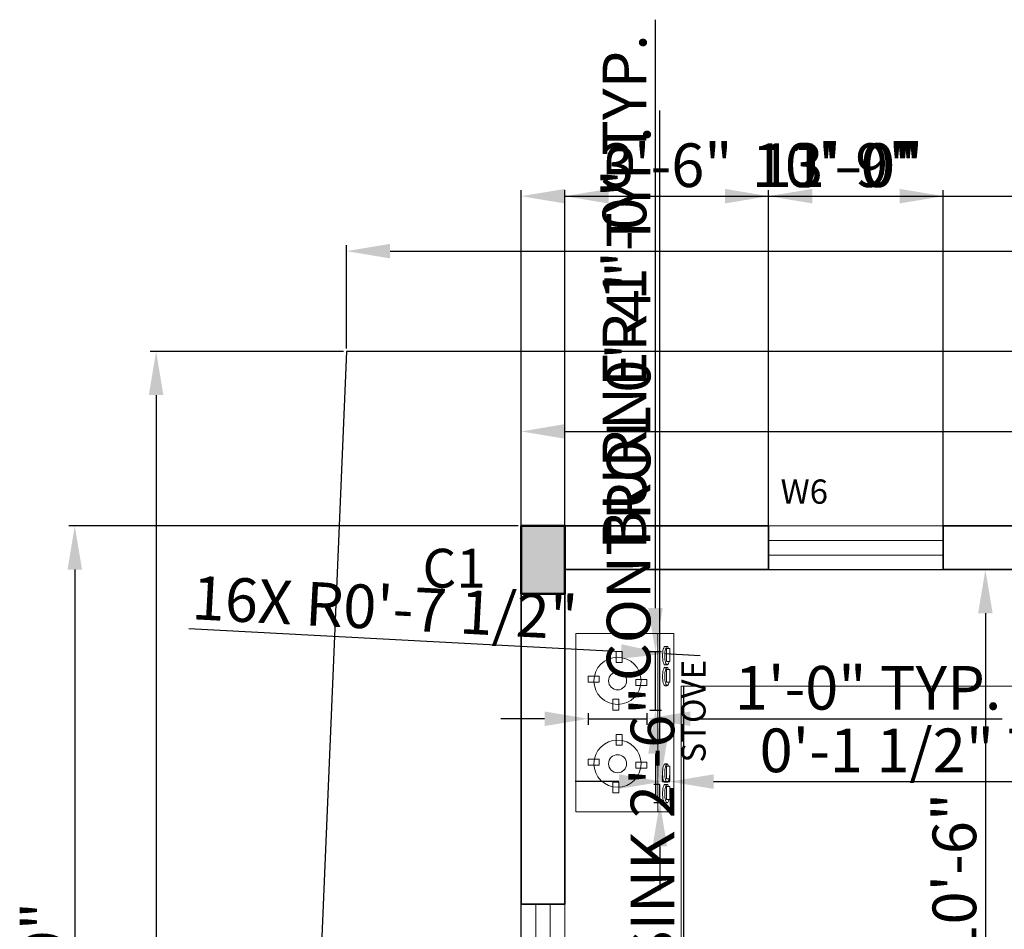
# Model space of a CAD drawing. Units: inches. Extents: x 2621 to 6190, y 513 to 1320.
# Tile 4 of 11: x 2675 to 2878, y 1003 to 1190. Entities that reach past the tile are written whole.
import ezdxf

# ---------------------------------------------------------------- set-up
doc = ezdxf.new("R2010")
doc.units = ezdxf.units.IN
for name, color, linetype, lineweight in [('A-ANNO-DIMS', 5, 'Continuous', 18), ('A-ANNO-TEXT', 7, 'Continuous', 18), ('A-EQPM', 30, 'Continuous', 13), ('A-FLOR-CASE', 30, 'Continuous', 18), ('A-WALL', 7, 'Continuous', 35), ('C-PROP', 7, 'Continuous', 25), ('columns', 2, 'Continuous', 50), ('S-COLS-IDEN', 2, 'Continuous', 25), ('S-COLS-PATT', 2, 'Continuous', 13), ('window', 172, 'Continuous', 18)]:
    doc.layers.add(name, color=color, linetype=linetype, lineweight=lineweight)
doc.styles.get("Standard").update_dxf_attribs({"font": 'arial.ttf'})
doc.dimstyles.new('ISO-25', dxfattribs={"dimtxt": 9, "dimasz": 9, "dimexe": 1.25, "dimexo": 0.625, "dimtad": 1, "dimlunit": 3, "dimtxsty": 'Standard', "dimcen": 2.5, "dimadec": 0, "dimazin": 0, "dimtfac": 1, "dimtmove": 0, "dimatfit": 3, "dimfxl": 1, "dimarcsym": 0})

# ---------------------------------------------------------------- blocks, each defined once
blk = doc.blocks.new('*D18')
at = {"layer": 'A-ANNO-DIMS', "color": 0, "lineweight": -2, "transparency": 16777216}
for p, q in [((2820.57, 1076.89), (2875.3, 1076.89)), ((2874.05, 1067.89), (2874.05, 959.89)), ((2820.57, 950.89), (2875.3, 950.89))]:
    blk.add_line(p, q, dxfattribs=at)
at = {"layer": 'A-ANNO-DIMS', "color": 0, "transparency": 16777216}
for points in [[(2872.55, 1067.89), (2875.55, 1067.89), (2874.05, 1076.89)], [(2872.55, 959.89), (2875.55, 959.89), (2874.05, 950.89)]]:
    blk.add_solid(points, dxfattribs=at)
at = {"layer": 'Defpoints', "color": 0, "transparency": 16777216}
for p in [(2819.94, 1076.89), (2819.94, 950.89), (2874.05, 950.89)]:
    blk.add_point(p, dxfattribs=at)
at = {"layer": 'A-ANNO-DIMS', "color": 0, "transparency": 16777216, "insert": (2868.83, 1013.89), "char_height": 9, "attachment_point": 5, "rotation": 90}
blk.add_mtext('10\'-6"', dxfattribs=at)
blk = doc.blocks.new('*D36')
at = {"layer": 'A-ANNO-DIMS', "color": 0, "lineweight": -2, "transparency": 16777216}
for p, q in [((2778.38, 1086.51), (2778.38, 1106.64)), ((3222.38, 1086.51), (3222.38, 1106.64)), ((2787.38, 1105.39), (3213.38, 1105.39))]:
    blk.add_line(p, q, dxfattribs=at)
at = {"layer": 'A-ANNO-DIMS', "color": 0, "transparency": 16777216}
for points in [[(2787.38, 1106.89), (2787.38, 1103.89), (2778.38, 1105.39)], [(3213.38, 1106.89), (3213.38, 1103.89), (3222.38, 1105.39)]]:
    blk.add_solid(points, dxfattribs=at)
at = {"layer": 'Defpoints', "color": 0, "transparency": 16777216}
for p in [(3222.38, 1105.39), (2778.38, 1085.89), (3222.38, 1085.89)]:
    blk.add_point(p, dxfattribs=at)
at = {"layer": 'A-ANNO-DIMS', "color": 0, "transparency": 16777216, "insert": (3000.38, 1110.61), "char_height": 9, "attachment_point": 5}
blk.add_mtext("37'", dxfattribs=at)
blk = doc.blocks.new('*D38')
at = {"layer": 'A-ANNO-DIMS', "color": 0, "lineweight": -2, "transparency": 16777216}
for p, q in [((2742.38, 1122.51), (2742.38, 1143.81)), ((2751.38, 1142.56), (3249.38, 1142.56)), ((3258.38, 1122.51), (3258.38, 1143.81))]:
    blk.add_line(p, q, dxfattribs=at)
at = {"layer": 'A-ANNO-DIMS', "color": 0, "transparency": 16777216}
for points in [[(2751.38, 1144.06), (2751.38, 1141.06), (2742.38, 1142.56)], [(3249.38, 1144.06), (3249.38, 1141.06), (3258.38, 1142.56)]]:
    blk.add_solid(points, dxfattribs=at)
at = {"layer": 'Defpoints', "color": 0, "transparency": 16777216}
for p in [(3258.38, 1142.56), (2742.38, 1121.89), (3258.38, 1121.89)]:
    blk.add_point(p, dxfattribs=at)
at = {"layer": 'A-ANNO-DIMS', "color": 0, "transparency": 16777216, "insert": (3000.38, 1147.79), "char_height": 9, "attachment_point": 5}
blk.add_mtext("43'", dxfattribs=at)
blk = doc.blocks.new('*D40')
at = {"layer": 'A-ANNO-DIMS', "color": 0, "lineweight": -2, "transparency": 16777216}
for p, q in [((2741.76, 1121.89), (2701.89, 1121.89)), ((2703.14, 1112.89), (2703.14, 561.89)), ((2717.76, 552.89), (2701.89, 552.89))]:
    blk.add_line(p, q, dxfattribs=at)
at = {"layer": 'A-ANNO-DIMS', "color": 0, "transparency": 16777216}
for points in [[(2701.64, 1112.89), (2704.64, 1112.89), (2703.14, 1121.89)], [(2701.64, 561.89), (2704.64, 561.89), (2703.14, 552.89)]]:
    blk.add_solid(points, dxfattribs=at)
at = {"layer": 'Defpoints', "color": 0, "transparency": 16777216}
for p in [(2742.38, 1121.89), (2703.14, 552.89), (2718.38, 552.89)]:
    blk.add_point(p, dxfattribs=at)
at = {"layer": 'A-ANNO-DIMS', "color": 0, "transparency": 16777216, "insert": (2697.94, 837.39), "char_height": 9, "attachment_point": 5, "rotation": 90}
blk.add_mtext('47\'-5"', dxfattribs=at)
blk = doc.blocks.new('WIN-VENT-24IN')
for p, q in [((9, 24), (0, 24)), ((0, 24), (0, 0)), ((3, 24), (3, 0)), ((6, 24), (6, 0)), ((9, 0), (9, 24)), ((0, 0), (9, 0))]:
    blk.add_line(p, q)
blk = doc.blocks.new('COOKTOP-BURNER')
for p, q in [((6.96, 12.04), (5.73, 12.04)), ((5.73, 12.04), (5.73, 9.81)), ((6.96, 9.81), (6.96, 12.04)), ((5.73, 9.81), (6.96, 9.81)), ((2.23, 6.96), (0, 6.96)), ((0, 6.96), (0, 5.73)), ((2.23, 5.73), (2.23, 6.96)), ((12.04, 6.31), (9.81, 6.31)), ((9.81, 6.31), (9.81, 5.08)), ((12.04, 5.08), (12.04, 6.31)), ((0, 5.73), (2.23, 5.73)), ((9.81, 5.08), (12.04, 5.08)), ((5.08, 2.23), (5.08, 0)), ((6.31, 2.23), (5.08, 2.23)), ((6.31, 0), (6.31, 2.23)), ((5.08, 0), (6.31, 0))]:
    blk.add_line(p, q)
for radius in [4.86, 1.86]:
    blk.add_circle((6.02, 6.02), radius)
blk = doc.blocks.new('COOKTOP-CONTROL')
for p, q in [((0.44, 3.79), (0.92, 3.78)), ((0.83, 3.35), (1.52, 3.35)), ((0.83, 0.69), (0.83, 3.35)), ((1.52, 3.35), (1.52, 0.69)), ((0.49, 0), (0.92, 0)), ((1.52, 0.69), (0.83, 0.69))]:
    blk.add_line(p, q)
for centre, radius, start, end in [((7.32, 1.89), 7.32, 173.9017, 180), ((3.91, 2.25), 3.89, 165.5369, 173.9017), ((1.79, 2.8), 1.7, 148.0894, 165.5369), ((0.49, 3.61), 0.166, 90, 148.0894), ((7.76, 1.89), 7.32, 173.9017, 180), ((4.35, 2.25), 3.89, 165.5369, 173.9017), ((0.49, 3.61), 0.166, 72.0546, 90), ((2.23, 2.8), 1.7, 148.0894, 165.5369), ((0.92, 3.61), 0.166, 90, 148.0894), ((0.92, 3.61), 0.166, 31.9106, 90), ((-0.38, 2.8), 1.7, 18.9155, 31.9106), ((7.32, 1.89), 7.32, 180, 186.0983), ((3.91, 1.53), 3.89, 186.0983, 194.4631), ((1.79, 0.98), 1.7, 194.4631, 211.9106), ((0.49, 0.17), 0.166, 211.9106, 270), ((7.76, 1.89), 7.32, 180, 186.0983), ((4.35, 1.53), 3.89, 186.0983, 194.4631), ((2.23, 0.98), 1.7, 194.4631, 211.9106), ((0.92, 0.17), 0.166, 211.9106, 270), ((0.92, 0.17), 0.166, 270, 328.0894), ((-0.38, 0.98), 1.7, 328.0894, 345.5369), ((-2.5, 1.53), 3.89, 345.5369, 347.5389)]:
    blk.add_arc(centre, radius, start, end)
blk = doc.blocks.new('*D67')
at = {"layer": 'A-ANNO-DIMS', "color": 0, "lineweight": -2, "transparency": 16777216}
for p, q in [((2806.96, 1041.61), (2806.96, 1171.58)), ((2806.9, 1032.61), (2805.71, 1032.61)), ((2806.96, 1028.83), (2806.96, 1032.61)), ((2806.9, 1028.83), (2805.71, 1028.83)), ((2806.96, 1019.83), (2806.96, 1010.83))]:
    blk.add_line(p, q, dxfattribs=at)
at = {"layer": 'A-ANNO-DIMS', "color": 0, "transparency": 16777216}
for points in [[(2805.46, 1041.61), (2808.46, 1041.61), (2806.96, 1032.61)], [(2805.46, 1019.83), (2808.46, 1019.83), (2806.96, 1028.83)]]:
    blk.add_solid(points, dxfattribs=at)
at = {"layer": 'Defpoints', "color": 0, "transparency": 16777216}
for p in [(2806.96, 1032.61), (2807.53, 1032.61), (2807.53, 1028.83)]:
    blk.add_point(p, dxfattribs=at)
at = {"layer": 'A-ANNO-DIMS', "color": 0, "transparency": 16777216, "insert": (2801.68, 1111.1), "char_height": 9, "attachment_point": 5, "rotation": 90}
blk.add_mtext('CONTROL 0\'-4" TYP.', dxfattribs=at)
blk = doc.blocks.new('*D68')
at = {"layer": 'A-ANNO-DIMS', "color": 0, "lineweight": -2, "transparency": 16777216}
for p, q in [((2798.53, 1033.18), (2789.53, 1033.18)), ((2807.53, 1033.24), (2807.53, 1034.43)), ((2807.53, 1033.18), (2809.04, 1033.18)), ((2809.04, 1033.24), (2809.04, 1034.43)), ((2818.04, 1033.18), (2904.12, 1033.18))]:
    blk.add_line(p, q, dxfattribs=at)
at = {"layer": 'A-ANNO-DIMS', "color": 0, "transparency": 16777216}
for points in [[(2798.53, 1034.68), (2798.53, 1031.68), (2807.53, 1033.18)], [(2818.04, 1034.68), (2818.04, 1031.68), (2809.04, 1033.18)]]:
    blk.add_solid(points, dxfattribs=at)
at = {"layer": 'Defpoints', "color": 0, "transparency": 16777216}
for p in [(2809.04, 1033.18), (2807.53, 1032.61), (2809.04, 1032.61)]:
    blk.add_point(p, dxfattribs=at)
at = {"layer": 'A-ANNO-DIMS', "color": 0, "transparency": 16777216, "insert": (2865.58, 1038.46), "char_height": 9, "attachment_point": 5}
blk.add_mtext('0\'-1 1/2" TYP.', dxfattribs=at)
blk = doc.blocks.new('*D69')
at = {"layer": 'A-ANNO-DIMS', "color": 0, "lineweight": -2, "transparency": 16777216}
for p, q in [((2806.06, 1068.98), (2806.06, 1190.28)), ((2804.88, 1059.98), (2807.31, 1059.98)), ((2806.06, 1047.94), (2806.06, 1059.98)), ((2804.88, 1047.94), (2807.31, 1047.94)), ((2806.06, 1038.94), (2806.06, 1029.94))]:
    blk.add_line(p, q, dxfattribs=at)
at = {"layer": 'A-ANNO-DIMS', "color": 0, "transparency": 16777216}
for points in [[(2804.56, 1068.98), (2807.56, 1068.98), (2806.06, 1059.98)], [(2804.56, 1038.94), (2807.56, 1038.94), (2806.06, 1047.94)]]:
    blk.add_solid(points, dxfattribs=at)
at = {"layer": 'Defpoints', "color": 0, "transparency": 16777216}
for p in [(2804.26, 1059.98), (2806.06, 1059.98), (2804.26, 1047.94)]:
    blk.add_point(p, dxfattribs=at)
at = {"layer": 'A-ANNO-DIMS', "color": 0, "transparency": 16777216, "insert": (2800.84, 1134.13), "char_height": 9, "attachment_point": 5, "rotation": 90}
blk.add_mtext('BURNER 1\'-0" TYP.', dxfattribs=at)
blk = doc.blocks.new('*D70')
at = {"layer": 'A-ANNO-DIMS', "color": 0, "lineweight": -2, "transparency": 16777216}
for p, q in [((2792.22, 1047.32), (2792.22, 1044.89)), ((2804.26, 1047.32), (2804.26, 1044.89)), ((2783.22, 1046.14), (2774.22, 1046.14)), ((2792.22, 1046.14), (2804.26, 1046.14)), ((2813.26, 1046.14), (2877.52, 1046.14))]:
    blk.add_line(p, q, dxfattribs=at)
at = {"layer": 'A-ANNO-DIMS', "color": 0, "transparency": 16777216}
for points in [[(2783.22, 1047.64), (2783.22, 1044.64), (2792.22, 1046.14)], [(2813.26, 1047.64), (2813.26, 1044.64), (2804.26, 1046.14)]]:
    blk.add_solid(points, dxfattribs=at)
at = {"layer": 'Defpoints', "color": 0, "transparency": 16777216}
for p in [(2792.22, 1047.94), (2804.26, 1047.94), (2804.26, 1046.14)]:
    blk.add_point(p, dxfattribs=at)
at = {"layer": 'A-ANNO-DIMS', "color": 0, "transparency": 16777216, "insert": (2849.89, 1051.36), "char_height": 9, "attachment_point": 5}
blk.add_mtext('1\'-0" TYP.', dxfattribs=at)
blk = doc.blocks.new('*D77')
at = {"layer": 'A-ANNO-DIMS', "color": 0, "lineweight": -2, "transparency": 16777216}
for p, q in [((2811.88, 985.99), (2811.88, 1052.96)), ((2808.01, 985.99), (2813.13, 985.99)), ((2811.88, 964.99), (2811.88, 976.99)), ((2808.01, 955.99), (2813.13, 955.99))]:
    blk.add_line(p, q, dxfattribs=at)
at = {"layer": 'A-ANNO-DIMS', "color": 0, "transparency": 16777216}
for points in [[(2810.38, 976.99), (2813.38, 976.99), (2811.88, 985.99)], [(2810.38, 964.99), (2813.38, 964.99), (2811.88, 955.99)]]:
    blk.add_solid(points, dxfattribs=at)
at = {"layer": 'Defpoints', "color": 0, "transparency": 16777216}
for p in [(2807.38, 985.99), (2811.88, 985.99), (2807.38, 955.99)]:
    blk.add_point(p, dxfattribs=at)
at = {"layer": 'A-ANNO-DIMS', "color": 0, "transparency": 16777216, "insert": (2806.6, 1023.98), "char_height": 9, "attachment_point": 5, "rotation": 90}
blk.add_mtext('SINK 2\'-6"', dxfattribs=at)
blk = doc.blocks.new('*D79')
at = {"layer": 'A-ANNO-DIMS', "color": 0, "lineweight": -2, "transparency": 16777216}
for p, q in [((2778.38, 1086.51), (2778.38, 1155.14)), ((2907.38, 1086.51), (2907.38, 1155.14)), ((2787.38, 1153.89), (2898.38, 1153.89))]:
    blk.add_line(p, q, dxfattribs=at)
at = {"layer": 'A-ANNO-DIMS', "color": 0, "transparency": 16777216}
for points in [[(2787.38, 1155.39), (2787.38, 1152.39), (2778.38, 1153.89)], [(2898.38, 1155.39), (2898.38, 1152.39), (2907.38, 1153.89)]]:
    blk.add_solid(points, dxfattribs=at)
at = {"layer": 'Defpoints', "color": 0, "transparency": 16777216}
for p in [(2907.38, 1153.89), (2778.38, 1085.89), (2907.38, 1085.89)]:
    blk.add_point(p, dxfattribs=at)
at = {"layer": 'A-ANNO-DIMS', "color": 0, "transparency": 16777216, "insert": (2842.88, 1159.11), "char_height": 9, "attachment_point": 5}
blk.add_mtext('10\'-9"', dxfattribs=at)
blk = doc.blocks.new('*D81')
at = {"layer": 'A-ANNO-DIMS', "color": 0, "lineweight": -2, "transparency": 16777216}
for p, q in [((2777.76, 1085.89), (2685.13, 1085.89)), ((2686.38, 1076.89), (2686.38, 905.89)), ((2777.76, 896.89), (2685.13, 896.89))]:
    blk.add_line(p, q, dxfattribs=at)
at = {"layer": 'A-ANNO-DIMS', "color": 0, "transparency": 16777216}
for points in [[(2684.88, 1076.89), (2687.88, 1076.89), (2686.38, 1085.89)], [(2684.88, 905.89), (2687.88, 905.89), (2686.38, 896.89)]]:
    blk.add_solid(points, dxfattribs=at)
at = {"layer": 'Defpoints', "color": 0, "transparency": 16777216}
for p in [(2778.38, 1085.89), (2686.38, 896.89), (2778.38, 896.89)]:
    blk.add_point(p, dxfattribs=at)
at = {"layer": 'A-ANNO-DIMS', "color": 0, "transparency": 16777216, "insert": (2681.16, 991.39), "char_height": 9, "attachment_point": 5, "rotation": 90}
blk.add_mtext('15\'-9"', dxfattribs=at)
blk = doc.blocks.new('*D87')
at = {"layer": 'A-ANNO-DIMS', "color": 0, "lineweight": -2, "transparency": 16777216}
for p, q in [((2778.38, 897.51), (2778.38, 1155.14)), ((2910.22, 898.87), (2910.22, 1155.14)), ((2787.38, 1153.89), (2901.22, 1153.89))]:
    blk.add_line(p, q, dxfattribs=at)
at = {"layer": 'A-ANNO-DIMS', "color": 0, "transparency": 16777216}
for points in [[(2787.38, 1155.39), (2787.38, 1152.39), (2778.38, 1153.89)], [(2901.22, 1155.39), (2901.22, 1152.39), (2910.22, 1153.89)]]:
    blk.add_solid(points, dxfattribs=at)
at = {"layer": 'Defpoints', "color": 0, "transparency": 16777216}
for p in [(2910.22, 1153.89), (2910.22, 898.24), (2778.38, 896.89)]:
    blk.add_point(p, dxfattribs=at)
at = {"layer": 'A-ANNO-DIMS', "color": 0, "transparency": 16777216, "insert": (2844.3, 1159.11), "char_height": 9, "attachment_point": 5}
blk.add_mtext('11\'-0"', dxfattribs=at)
blk = doc.blocks.new('*D104')
at = {"layer": 'A-ANNO-DIMS', "color": 0, "lineweight": -2, "transparency": 16777216}
for p, q in [((2829.38, 1077.51), (2829.38, 1155.14)), ((2865.38, 1077.51), (2865.38, 1155.14)), ((2838.38, 1153.89), (2856.38, 1153.89))]:
    blk.add_line(p, q, dxfattribs=at)
at = {"layer": 'A-ANNO-DIMS', "color": 0, "transparency": 16777216}
for points in [[(2838.38, 1155.39), (2838.38, 1152.39), (2829.38, 1153.89)], [(2856.38, 1155.39), (2856.38, 1152.39), (2865.38, 1153.89)]]:
    blk.add_solid(points, dxfattribs=at)
at = {"layer": 'Defpoints', "color": 0, "transparency": 16777216}
for p in [(2865.38, 1153.89), (2829.38, 1076.89), (2865.38, 1076.89)]:
    blk.add_point(p, dxfattribs=at)
at = {"layer": 'A-ANNO-DIMS', "color": 0, "transparency": 16777216, "insert": (2847.38, 1159.11), "char_height": 9, "attachment_point": 5}
blk.add_mtext('3\'-0"', dxfattribs=at)
blk = doc.blocks.new('*D105')
at = {"layer": 'A-ANNO-DIMS', "color": 0, "lineweight": -2, "transparency": 16777216}
for p, q in [((2787.38, 1077.51), (2787.38, 1155.14)), ((2829.38, 1077.51), (2829.38, 1155.14)), ((2796.38, 1153.89), (2820.38, 1153.89))]:
    blk.add_line(p, q, dxfattribs=at)
at = {"layer": 'A-ANNO-DIMS', "color": 0, "transparency": 16777216}
for points in [[(2796.38, 1155.39), (2796.38, 1152.39), (2787.38, 1153.89)], [(2820.38, 1155.39), (2820.38, 1152.39), (2829.38, 1153.89)]]:
    blk.add_solid(points, dxfattribs=at)
at = {"layer": 'Defpoints', "color": 0, "transparency": 16777216}
for p in [(2829.38, 1153.89), (2787.38, 1076.89), (2829.38, 1076.89)]:
    blk.add_point(p, dxfattribs=at)
at = {"layer": 'A-ANNO-DIMS', "color": 0, "transparency": 16777216, "insert": (2808.38, 1159.11), "char_height": 9, "attachment_point": 5}
blk.add_mtext('3\'-6"', dxfattribs=at)
blk = doc.blocks.new('*D117')
at = {"layer": 'A-ANNO-DIMS', "color": 0, "lineweight": -2, "transparency": 16777216}
for p, q in [((2709.87, 1064.76), (2798.98, 1060.02)), ((2815.28, 1059.15), (2807.97, 1059.54))]:
    blk.add_line(p, q, dxfattribs=at)
at = {"layer": 'A-ANNO-DIMS', "color": 0, "transparency": 16777216}
blk.add_solid([(2799.06, 1061.51), (2798.9, 1058.52), (2807.97, 1059.54)], dxfattribs=at)
at = {"layer": 'Defpoints', "color": 0, "transparency": 16777216}
for p in [(2807.97, 1059.54), (2815.28, 1059.15)]:
    blk.add_point(p, dxfattribs=at)
at = {"layer": 'A-ANNO-DIMS', "color": 0, "transparency": 16777216, "insert": (2750.21, 1067.9), "char_height": 9, "attachment_point": 5, "rotation": 356.9538}
blk.add_mtext('16X R0\'-7 1/2"', dxfattribs=at)

msp = doc.modelspace()

# ---------------------------------------------------------------- hatches: boundary and pattern name
at = {"layer": 'S-COLS-PATT'}
h = msp.add_hatch(color=256, dxfattribs=at)
h.dxf.hatch_style = 1
h.paths.add_polyline_path([(2787.381, 1085.89), (2778.381, 1085.89), (2778.381, 1071.89), (2787.381, 1071.89)])
h.paths.add_polyline_path([(3222.381, 1085.89), (3208.381, 1085.89), (3208.381, 1076.89), (3222.381, 1076.89)])
h.paths.add_polyline_path([(3041.381, 1085.89), (3027.381, 1085.89), (3027.381, 1076.89), (3041.381, 1076.89)])
h.paths.add_polyline_path([(2916.381, 1085.89), (2907.381, 1085.89), (2907.381, 1076.89), (2916.381, 1076.89)])
h.paths.add_polyline_path([(2916.381, 1076.89), (2913.381, 1076.89), (2913.381, 1071.89), (2916.381, 1071.89)])
h.paths.add_polyline_path([(2913.381, 1076.89), (2907.381, 1076.89), (2907.381, 1071.89), (2913.381, 1071.89)])
h.paths.add_polyline_path([(2787.381, 896.89), (2778.381, 896.89), (2778.381, 882.89), (2787.381, 882.89)])
h.paths.add_polyline_path([(2924.221, 898.241), (2910.221, 898.241), (2910.221, 889.241), (2924.221, 889.241)])
h.paths.add_polyline_path([(3036.381, 896.89), (3033.381, 896.89), (3027.381, 897.385), (3027.381, 883.385), (3033.381, 883.385), (3033.381, 890.89), (3036.381, 890.89)])
h.paths.add_polyline_path([(3036.381, 890.89), (3033.381, 890.89), (3033.381, 883.385), (3036.381, 883.385)], flags=17)
h.paths.add_polyline_path([(3222.381, 897.745), (3213.381, 897.745), (3213.381, 883.745), (3222.381, 883.745)])
h.paths.add_polyline_path([(3222.381, 710.89), (3208.381, 710.89), (3208.381, 701.89), (3222.381, 701.89)])
h.paths.add_polyline_path([(3039.318, 710.89), (3021.318, 710.89), (3021.318, 701.89), (3039.318, 701.89)])
h.paths.add_polyline_path([(2796.381, 710.89), (2778.381, 710.89), (2778.381, 701.89), (2796.381, 701.89)])

# ---------------------------------------------------------------- linework, layer by layer
at = {"layer": 'A-EQPM'}
for p, q in [((2789.665, 1063.691), (2809.848, 1063.691)), ((2789.665, 1026.986), (2789.665, 1063.691)), ((2806.566, 1063.691), (2806.566, 1026.986)), ((2809.848, 1063.691), (2809.848, 1026.986)), ((2809.848, 1026.986), (2789.665, 1026.986))]:
    msp.add_line(p, q, dxfattribs=at)
at = {"layer": 'A-FLOR-CASE'}
for p, q in [((2811.381, 1052.89), (2811.381, 950.89)), ((2907.381, 1052.89), (2811.381, 1052.89))]:
    msp.add_line(p, q, dxfattribs=at)
at = {"layer": 'A-WALL'}
for p, q in [((2778.381, 1085.89), (2778.381, 1007.89)), ((2829.381, 1085.89), (2778.381, 1085.89)), ((2829.381, 1076.89), (2829.381, 1085.89)), ((2865.381, 1076.89), (2865.381, 1085.89)), ((2949.381, 1085.89), (2865.381, 1085.89)), ((2787.381, 1076.89), (2787.381, 1007.89)), ((2829.381, 1076.89), (2787.381, 1076.89)), ((2907.381, 1076.89), (2865.381, 1076.89)), ((2787.381, 1007.89), (2778.381, 1007.89))]:
    msp.add_line(p, q, dxfattribs=at)
at = {"layer": 'C-PROP'}
msp.add_lwpolyline([(3258.381, 552.89), (3258.381, 1121.89), (2742.381, 1121.89), (2718.381, 552.89)], close=True, dxfattribs=at)
at = {"layer": 'columns'}
msp.add_lwpolyline([(2778.381, 1085.89), (2787.381, 1085.89), (2787.381, 1071.89), (2778.381, 1071.89)], close=True, dxfattribs=at)
at = {"layer": 'window'}
for p, q in [((2865.381, 1085.89), (2829.381, 1085.89)), ((2829.381, 1085.89), (2829.381, 1076.89)), ((2865.381, 1076.89), (2865.381, 1085.89)), ((2829.381, 1082.89), (2865.381, 1082.89)), ((2829.381, 1079.89), (2865.381, 1079.89)), ((2829.381, 1076.89), (2865.381, 1076.89))]:
    msp.add_line(p, q, dxfattribs=at)

# ---------------------------------------------------------------- block references
at = {"layer": 'A-EQPM'}
for name, p in [('COOKTOP-BURNER', (2792.218, 1047.944)), ('COOKTOP-CONTROL', (2807.526, 1057.258)), ('COOKTOP-CONTROL', (2807.526, 1052.966)), ('COOKTOP-CONTROL', (2807.526, 1033.039)), ('COOKTOP-CONTROL', (2807.526, 1028.829))]:
    msp.add_blockref(name, p, dxfattribs=at)
at = {"layer": 'A-EQPM', "rotation": 180}
msp.add_blockref('COOKTOP-BURNER', (2804.258, 1042.896), dxfattribs=at)
at = {"layer": 'window'}
msp.add_blockref('WIN-VENT-24IN', (2778.381, 983.89), dxfattribs=at)

# ---------------------------------------------------------------- texts
at = {"layer": 'A-ANNO-TEXT', "insert": (2831.846, 1095.476), "char_height": 5, "attachment_point": 1}
msp.add_mtext_dynamic_manual_height_columns('W6', width=21.64382, gutter_width=12.5, heights=[0], dxfattribs=at)
at = {"layer": 'A-ANNO-TEXT', "insert": (2811.381, 1037.116), "char_height": 5, "attachment_point": 1, "rotation": 90}
msp.add_mtext_dynamic_manual_height_columns('STOVE', width=26.0401, gutter_width=12.5, heights=[0], dxfattribs=at)
at = {"layer": 'S-COLS-IDEN', "insert": (2758.043, 1081.182), "char_height": 8, "attachment_point": 1}
msp.add_mtext_dynamic_manual_height_columns('C1', width=53.01391, gutter_width=12.5, heights=[0], dxfattribs=at)

# ---------------------------------------------------------------- dimensions: what is measured, and where the dimension line sits
at = {"layer": 'A-ANNO-DIMS'}
for base, p1, p2, text, picture, middle in [((2806.063, 1059.984), (2804.258, 1047.944), (2804.258, 1059.984), 'BURNER <> TYP.', '*D69', (2800.843, 1134.131)), ((2806.958, 1032.614), (2807.526, 1028.829), (2807.526, 1032.614), 'CONTROL <> TYP.', '*D67', (2801.676, 1111.099)), ((2811.881, 985.99), (2807.381, 955.99), (2807.381, 985.99), 'SINK <>', '*D77', (2806.603, 1023.975))]:
    dim = msp.add_linear_dim(base=base, p1=p1, p2=p2, angle=90, text=text, dimstyle='ISO-25', override={"dimdec": 1, "dimlfac": 1, "dimrnd": 0, "dimzin": 1, "dimdsep": 46, "dimlunit": 4, "dimfrac": 2}, dxfattribs=at)
    dim.commit()
    dim.dimension.update_dxf_attribs({"geometry": picture, "text_midpoint": middle})
for base, p1, p2, override, picture, middle in [((2907.381, 1153.89), (2778.381, 1085.89), (2907.381, 1085.89), {"dimdec": 1, "dimlfac": 1, "dimrnd": 0, "dimzin": 1, "dimdsep": 46, "dimlunit": 4, "dimfrac": 2}, '*D79', (2842.881, 1159.11)), ((2910.221, 1153.89), (2778.381, 896.89), (2910.221, 898.241), {"dimdec": 1, "dimlfac": 1, "dimrnd": 0, "dimzin": 1, "dimdsep": 46, "dimlunit": 4, "dimfrac": 2}, '*D87', (2844.301, 1159.11)), ((2829.381, 1153.89), (2787.381, 1076.89), (2829.381, 1076.89), {"dimdec": 1, "dimlfac": 1, "dimrnd": 0, "dimzin": 1, "dimdsep": 46, "dimlunit": 4, "dimfrac": 2}, '*D105', (2808.381, 1159.113)), ((2865.381, 1153.89), (2829.381, 1076.89), (2865.381, 1076.89), {"dimdec": 1, "dimlfac": 1, "dimrnd": 0, "dimzin": 1, "dimdsep": 46, "dimlunit": 4, "dimfrac": 2}, '*D104', (2847.381, 1159.113)), ((3258.381, 1142.564), (2742.381, 1121.89), (3258.381, 1121.89), {"dimclrd": 0, "dimclre": 0, "dimclrt": 0}, '*D38', (3000.381, 1147.788)), ((3222.381, 1105.387), (2778.381, 1085.89), (3222.381, 1085.89), {"dimclrd": 0, "dimclre": 0, "dimclrt": 0}, '*D36', (3000.381, 1110.61))]:
    dim = msp.add_linear_dim(base=base, p1=p1, p2=p2, dimstyle='ISO-25', override=override, dxfattribs=at)
    dim.commit()
    dim.dimension.update_dxf_attribs({"geometry": picture, "text_midpoint": middle})
for base, p1, p2, override, picture, middle in [((2703.139, 552.89), (2742.381, 1121.89), (2718.381, 552.89), {"dimclrd": 0, "dimclre": 0, "dimclrt": 0}, '*D40', (2697.937, 837.39)), ((2686.381, 896.89), (2778.381, 1085.89), (2778.381, 896.89), {"dimdec": 1, "dimlfac": 1, "dimrnd": 0, "dimzin": 1, "dimdsep": 46, "dimlunit": 4, "dimfrac": 2}, '*D81', (2681.161, 991.39)), ((2874.051, 950.89), (2819.945, 1076.89), (2819.945, 950.89), {"dimclrd": 0, "dimclre": 0, "dimclrt": 0}, '*D18', (2868.831, 1013.89))]:
    dim = msp.add_linear_dim(base=base, p1=p1, p2=p2, angle=90, dimstyle='ISO-25', override=override, dxfattribs=at)
    dim.commit()
    dim.dimension.update_dxf_attribs({"geometry": picture, "text_midpoint": middle})
dim = msp.add_radius_dim(center=(2815.281, 1059.149), mpoint=(2807.97, 1059.538), text='16X <>', dimstyle='ISO-25', override={"dimdec": 1, "dimlfac": 1, "dimrnd": 0, "dimzin": 1, "dimdsep": 46, "dimlunit": 4, "dimfrac": 2}, dxfattribs=at)
dim.commit()
dim.dimension.update_dxf_attribs({"geometry": '*D117', "text_midpoint": (2750.211, 1067.898)})
for base, p1, p2, picture, middle in [((2804.258, 1046.138), (2792.218, 1047.944), (2804.258, 1047.944), '*D70', (2849.889, 1051.358)), ((2809.041, 1033.182), (2807.526, 1032.614), (2809.041, 1032.614), '*D68', (2865.582, 1038.461))]:
    dim = msp.add_linear_dim(base=base, p1=p1, p2=p2, text='<> TYP.', dimstyle='ISO-25', override={"dimdec": 1, "dimlfac": 1, "dimrnd": 0, "dimzin": 1, "dimdsep": 46, "dimlunit": 4, "dimfrac": 2}, dxfattribs=at)
    dim.commit()
    dim.dimension.update_dxf_attribs({"geometry": picture, "text_midpoint": middle})

doc.saveas('drawing.dxf')
